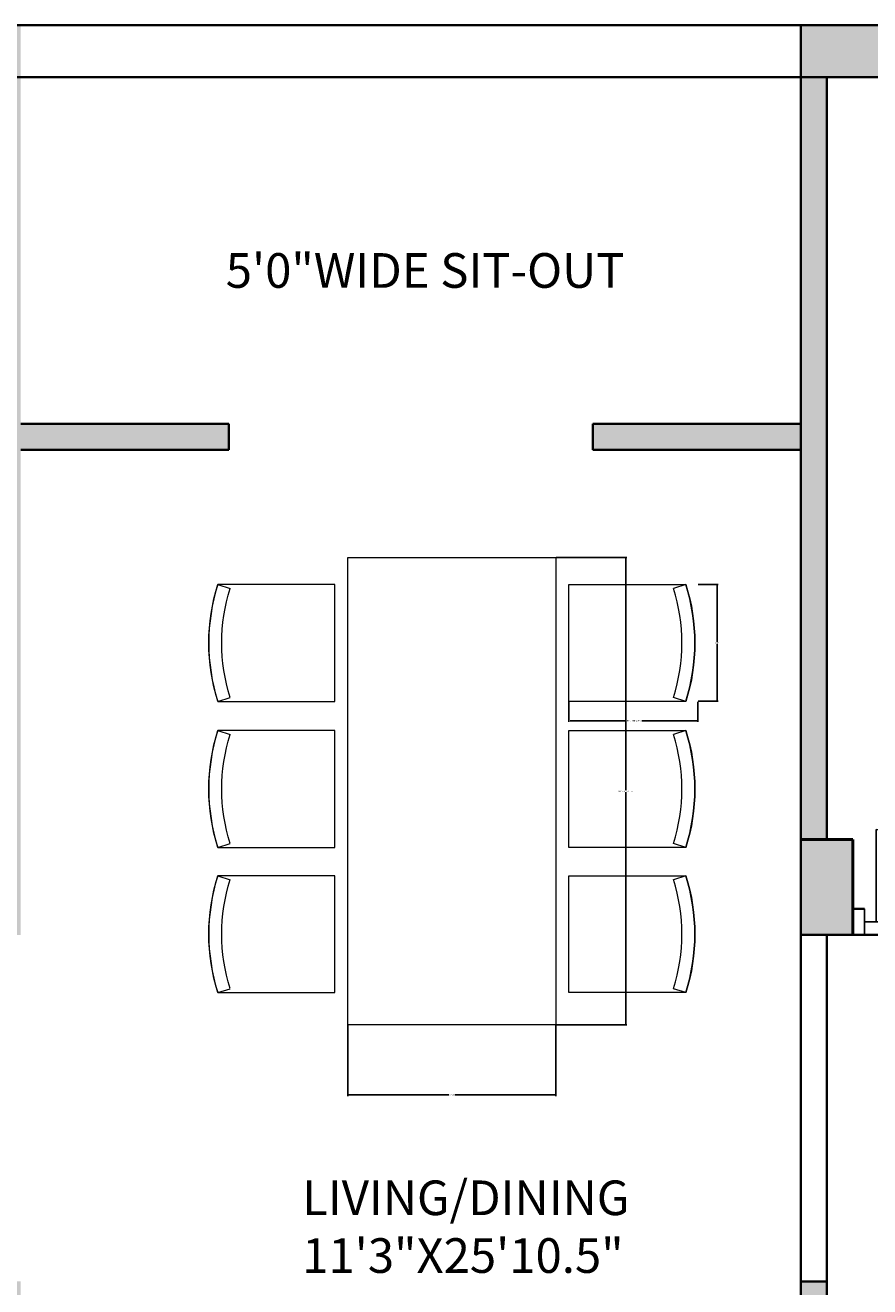
# Model space of a CAD drawing. Units: inches. Extents: x -28 to 485, y -861 to 54.
# Tile 12 of 14: x 162 to 308, y -208 to 10. Entities that reach past the tile are written whole.
import ezdxf

# ---------------------------------------------------------------- set-up
doc = ezdxf.new("R2010")
doc.units = ezdxf.units.IN
doc.header["$MEASUREMENT"] = 0
for name, color, linetype, lineweight in [('A-ANNO-DIMS', 2, 'Continuous', 18), ('A-AREA-IDEN', 7, 'Continuous', 18), ('A-COLS', 7, 'Continuous', 50), ('A-COLS-PATT', 8, 'Continuous', 13), ('A-DOOR', 3, 'Continuous', 25), ('A-FURN', 8, 'Continuous', 13), ('A-WALL', 7, 'Continuous', 35), ('A-WALL-PATT', 34, 'Continuous', 13)]:
    doc.layers.add(name, color=color, linetype=linetype, lineweight=lineweight)
doc.styles.get("Standard").update_dxf_attribs({"font": 'arial.ttf'})
doc.dimstyles.get("Standard").update_dxf_attribs({"dimtxt": 0.18, "dimasz": 0.18, "dimexe": 0.18, "dimexo": 0.0625, "dimgap": 0.09, "dimtad": 0, "dimtih": 1, "dimtoh": 1, "dimdec": 0, "dimzin": 0, "dimdsep": 46, "dimlunit": 3, "dimtxsty": 'Standard', "dimcen": 0.09, "dimadec": 0, "dimazin": 0, "dimtfac": 1, "dimtdec": 0, "dimtofl": 0, "dimtmove": 0, "dimatfit": 3, "dimfxl": 1, "dimtolj": 1, "dimtzin": 0, "dimarcsym": 0})

# ---------------------------------------------------------------- blocks, each defined once
blk = doc.blocks.new('CHAIR-DINING')
for p, q in [((20.22, 20.23), (18.08, 19.55)), ((20.22, 0), (18.08, 0.68))]:
    blk.add_line(p, q)
blk.add_lwpolyline([(20.23, 0), (0, 0), (0, 20.23), (20.23, 20.23, -0.153703), (20.23, 0)], format="xyb")
for radius in [33.37, 31.13]:
    blk.add_arc((-11.59, 10.12), radius, 342.3544, 17.6456)
blk = doc.blocks.new('TABLE-DINING-RECT')
blk.add_lwpolyline([(0, 80.93), (35.97, 80.93), (35.97, 0), (0, 0)], close=True)
blk = doc.blocks.new('DOOR-SWING-NARROW')
for p, q in [((17, 2.25), (17, 18.25)), ((18, 2.25), (18, 18.25)), ((0, 2.25), (0, 4.5)), ((20, 4.5), (20, 0)), ((0, 2.25), (0, 0)), ((0, 2.25), (2, 2.25)), ((17, 2.25), (18, 2.25)), ((20, 2.25), (18, 2.25))]:
    blk.add_line(p, q)
blk.add_arc((18, 2.25), 16, 90, 180)
blk = doc.blocks.new('*D18')
at = {"layer": 'A-ANNO-DIMS', "color": 0, "lineweight": -2, "transparency": 16777216}
for p, q in [((255.64, -107), (255.64, -110.46)), ((277.95, -107), (277.95, -110.46)), ((255.82, -110.28), (265.37, -110.28)), ((277.77, -110.28), (268.22, -110.28))]:
    blk.add_line(p, q, dxfattribs=at)
at = {"layer": 'A-ANNO-DIMS', "color": 0, "transparency": 16777216}
for points in [[(255.82, -110.25), (255.82, -110.31), (255.64, -110.28)], [(277.77, -110.25), (277.77, -110.31), (277.95, -110.28)]]:
    blk.add_solid(points, dxfattribs=at)
at = {"layer": 'Defpoints', "color": 0, "transparency": 16777216}
for p in [(255.64, -106.93), (277.95, -106.93), (277.95, -110.28)]:
    blk.add_point(p, dxfattribs=at)
at = {"layer": 'A-ANNO-DIMS', "color": 0, "transparency": 16777216, "insert": (266.8, -110.28), "char_height": 0.18, "attachment_point": 5}
blk.add_mtext('\\A1;DINING CHAIR 22 TYP.', dxfattribs=at)
blk = doc.blocks.new('*D19')
at = {"layer": 'A-ANNO-DIMS', "color": 0, "lineweight": -2, "transparency": 16777216}
for p, q in [((278.01, -86.7), (281.48, -86.7)), ((281.3, -86.88), (281.3, -96.63)), ((281.3, -106.75), (281.3, -97)), ((278.01, -106.93), (281.48, -106.93))]:
    blk.add_line(p, q, dxfattribs=at)
at = {"layer": 'A-ANNO-DIMS', "color": 0, "transparency": 16777216}
for points in [[(281.27, -86.88), (281.33, -86.88), (281.3, -86.7)], [(281.27, -106.75), (281.33, -106.75), (281.3, -106.93)]]:
    blk.add_solid(points, dxfattribs=at)
at = {"layer": 'Defpoints', "color": 0, "transparency": 16777216}
for p in [(277.95, -86.7), (281.3, -86.7), (277.95, -106.93)]:
    blk.add_point(p, dxfattribs=at)
at = {"layer": 'A-ANNO-DIMS', "color": 0, "transparency": 16777216, "insert": (281.3, -96.82), "char_height": 0.18, "attachment_point": 5}
blk.add_mtext('\\A1;20 TYP.', dxfattribs=at)
blk = doc.blocks.new('*D42')
at = {"layer": 'A-ANNO-DIMS', "color": 0, "lineweight": -2, "transparency": 16777216}
for p, q in [((253.42, -82.02), (265.67, -82.02)), ((265.49, -82.2), (265.49, -122.3)), ((265.49, -162.77), (265.49, -122.67)), ((253.42, -162.95), (265.67, -162.95))]:
    blk.add_line(p, q, dxfattribs=at)
at = {"layer": 'A-ANNO-DIMS', "color": 0, "transparency": 16777216}
for points in [[(265.46, -82.2), (265.52, -82.2), (265.49, -82.02)], [(265.46, -162.77), (265.52, -162.77), (265.49, -162.95)]]:
    blk.add_solid(points, dxfattribs=at)
at = {"layer": 'Defpoints', "color": 0, "transparency": 16777216}
for p in [(253.35, -82.02), (265.49, -82.02), (253.35, -162.95)]:
    blk.add_point(p, dxfattribs=at)
at = {"layer": 'A-ANNO-DIMS', "color": 0, "transparency": 16777216, "insert": (265.49, -122.48), "char_height": 0.18, "attachment_point": 5}
blk.add_mtext('\\A1;DINING TABLE 81 TYP.', dxfattribs=at)
blk = doc.blocks.new('*D43')
at = {"layer": 'A-ANNO-DIMS', "color": 0, "lineweight": -2, "transparency": 16777216}
for p, q in [((217.38, -163.01), (217.38, -175.27)), ((253.35, -163.01), (253.35, -175.27)), ((217.56, -175.09), (234.84, -175.09)), ((253.17, -175.09), (235.9, -175.09))]:
    blk.add_line(p, q, dxfattribs=at)
at = {"layer": 'A-ANNO-DIMS', "color": 0, "transparency": 16777216}
for points in [[(217.56, -175.06), (217.56, -175.12), (217.38, -175.09)], [(253.17, -175.06), (253.17, -175.12), (253.35, -175.09)]]:
    blk.add_solid(points, dxfattribs=at)
at = {"layer": 'Defpoints', "color": 0, "transparency": 16777216}
for p in [(217.38, -162.95), (253.35, -162.95), (253.35, -175.09)]:
    blk.add_point(p, dxfattribs=at)
at = {"layer": 'A-ANNO-DIMS', "color": 0, "transparency": 16777216, "insert": (235.37, -175.09), "char_height": 0.18, "attachment_point": 5}
blk.add_mtext('\\A1;36 TYP.', dxfattribs=at)

msp = doc.modelspace()

# ---------------------------------------------------------------- hatches: boundary and pattern name
at = {"layer": 'A-COLS-PATT'}
h = msp.add_hatch(color=256, dxfattribs=at)
h.dxf.hatch_style = 1
h.paths.add_polyline_path([(36.285, 10.133), (15.285, 10.133), (15.285, 1.133), (36.285, 1.133)])
h.paths.add_polyline_path([(160.785, 10.133), (139.785, 10.133), (139.785, 1.133), (160.785, 1.133)])
h.paths.add_polyline_path([(316.785, 10.133), (295.785, 10.133), (295.785, 1.133), (316.785, 1.133)])
h.paths.add_polyline_path([(441.285, 10.133), (420.285, 10.133), (420.285, 1.133), (441.285, 1.133)])
h.paths.add_polyline_path([(441.285, -138.367), (432.285, -138.367), (420.285, -138.367), (420.285, -147.367), (441.285, -147.367)])
h.paths.add_polyline_path([(304.785, -130.867), (295.785, -130.867), (295.785, -147.367), (304.785, -147.367), (304.785, -142.867)])
h.paths.add_polyline_path([(160.785, -130.867), (151.785, -130.867), (151.785, -142.867), (151.785, -147.367), (160.785, -147.367)])
h.paths.add_polyline_path([(36.285, -138.367), (24.285, -138.367), (15.285, -138.367), (15.285, -147.367), (36.285, -147.367)])
h.paths.add_polyline_path([(36.285, -355.867), (15.285, -355.867), (15.285, -364.867), (36.285, -364.867)])
h.paths.add_polyline_path([(160.785, -355.867), (139.785, -355.867), (139.785, -364.867), (160.785, -364.867)])
h.paths.add_polyline_path([(316.785, -355.867), (300.285, -355.867), (295.785, -355.867), (295.785, -364.867), (316.785, -364.867)])
at = {"layer": 'A-WALL-PATT'}
h = msp.add_hatch(color=256, dxfattribs=at)
h.dxf.hatch_style = 1
h.paths.add_polyline_path([(160.785, -808.867), (160.785, -817.867), (295.785, -817.867), (295.785, -808.867)])
h.paths.add_polyline_path([(316.785, -817.867), (323.776, -817.867), (323.776, -808.867), (316.785, -808.867)])
h.paths.add_polyline_path([(420.285, -817.867), (420.285, -808.867), (383.776, -808.867), (383.776, -817.867)])
h.paths.add_polyline_path([(432.285, -808.867), (441.285, -808.867), (441.285, -702.966), (432.285, -702.966), (432.285, -708.367), (397.785, -708.367), (397.785, -710.617), (397.785, -712.867), (432.285, -712.867)])
h.paths.add_polyline_path([(300.285, -712.867), (329.285, -712.867), (329.285, -710.617), (329.285, -708.367), (295.785, -708.367), (295.785, -808.867), (300.285, -808.867)])
h.paths.add_polyline_path([(160.785, -698.867), (158.535, -698.867), (156.285, -698.867), (156.285, -808.867), (160.785, -808.867)])
h.paths.add_polyline_path([(36.285, -808.867), (36.285, -817.867), (79.721, -817.867), (79.721, -808.867)])
h.paths.add_polyline_path([(15.285, -808.867), (24.285, -808.867), (24.285, -739.09), (15.285, -739.09)])
h.paths.add_polyline_path([(24.285, -640.781), (15.285, -640.781), (15.285, -679.09), (24.285, -679.09), (24.285, -664.867), (89.285, -664.867), (89.285, -662.617), (89.285, -660.367), (24.285, -660.367)])
h.paths.add_polyline_path([(15.285, -616.781), (24.285, -616.781), (24.285, -600.367), (15.285, -600.367)])
h.paths.add_polyline_path([(36.285, -595.867), (36.285, -600.367), (123.285, -600.367), (123.285, -660.367), (117.285, -660.367), (117.285, -664.867), (156.285, -664.867), (156.285, -670.867), (160.785, -670.867), (160.785, -660.367), (127.785, -660.367), (127.785, -600.367), (129.785, -600.367), (129.785, -598.117), (129.785, -595.867)])
h.paths.add_polyline_path([(367.785, -664.867), (363.285, -664.867), (363.285, -708.367), (357.285, -708.367), (357.285, -712.867), (369.785, -712.867), (369.785, -708.367), (367.785, -708.367)])
h.paths.add_polyline_path([(432.285, -664.867), (432.285, -666.966), (441.285, -666.966), (441.285, -642.367), (432.285, -642.367), (432.285, -660.367), (328.785, -660.367), (328.785, -664.867), (363.285, -664.867)])
h.paths.add_polyline_path([(333.285, -600.367), (420.285, -600.367), (420.285, -595.867), (326.785, -595.867), (326.785, -600.367), (328.785, -600.367), (328.785, -630.367), (331.035, -630.367), (333.285, -630.367)])
h.paths.add_polyline_path([(441.285, -600.367), (432.285, -600.367), (432.285, -618.367), (441.285, -618.367)])
h.paths.add_polyline_path([(432.285, -591.367), (441.285, -591.367), (441.285, -547.793), (432.285, -547.793)])
h.paths.add_polyline_path([(295.785, -588.367), (300.238, -588.367), (300.285, -583.867), (300.285, -451.867), (295.785, -451.867)])
h.paths.add_polyline_path([(420.285, -451.867), (420.285, -442.867), (316.785, -442.867), (316.785, -451.867)])
h.paths.add_polyline_path([(432.285, -487.793), (441.285, -487.793), (441.285, -451.867), (432.285, -451.867)])
h.paths.add_polyline_path([(432.285, -442.867), (441.285, -442.867), (441.285, -364.867), (432.285, -364.867)])
h.paths.add_polyline_path([(261.785, -451.867), (261.785, -447.367), (261.785, -444.758), (261.785, -442.867), (160.785, -442.867), (160.785, -451.867)])
h.paths.add_polyline_path([(139.785, -451.867), (139.785, -442.867), (36.285, -442.867), (36.285, -451.867)])
h.paths.add_polyline_path([(15.285, -491.617), (24.285, -491.617), (24.285, -451.867), (15.285, -451.867)])
h.paths.add_polyline_path([(24.285, -551.617), (15.285, -551.617), (15.285, -591.367), (24.285, -591.367)])
h.paths.add_polyline_path([(160.785, -451.867), (156.285, -451.867), (156.285, -588.367), (160.785, -588.367)])
h.paths.add_polyline_path([(139.785, -364.867), (139.785, -355.867), (36.285, -355.867), (36.285, -364.867)])
h.paths.add_polyline_path([(24.285, -364.867), (15.285, -364.867), (15.285, -373.867), (24.285, -373.867)])
h.paths.add_polyline_path([(15.285, -433.867), (15.285, -442.867), (24.285, -442.867), (24.285, -433.867)])
h.paths.add_polyline_path([(261.785, -364.867), (261.785, -360.367), (261.785, -355.867), (160.785, -355.867), (160.785, -364.867)])
h.paths.add_polyline_path([(295.785, -355.867), (289.785, -355.867), (289.785, -364.867), (295.785, -364.867)])
h.paths.add_polyline_path([(295.785, -355.867), (300.285, -355.867), (300.285, -259.867), (333.285, -259.867), (333.285, -257.617), (333.285, -255.367), (300.285, -255.367), (300.285, -207.367), (295.785, -207.367)])
h.paths.add_polyline_path([(420.285, -364.867), (420.285, -355.867), (316.785, -355.867), (316.785, -364.867)])
h.paths.add_polyline_path([(24.285, -311.192), (15.285, -311.192), (15.285, -355.867), (24.285, -355.867)])
h.paths.add_polyline_path([(24.285, -211.867), (54.144, -211.867), (54.144, -207.367), (24.285, -207.367), (24.285, -187.772), (15.285, -187.772), (15.285, -251.192), (24.285, -251.192)])
h.paths.add_polyline_path([(82.144, -207.367), (82.144, -209.617), (82.144, -211.867), (127.785, -211.867), (127.785, -147.367), (129.785, -147.367), (129.785, -145.117), (129.785, -142.867), (36.285, -142.867), (36.285, -147.367), (123.285, -147.367), (123.285, -207.367)])
h.paths.add_polyline_path([(160.785, -207.367), (156.285, -207.367), (156.285, -355.867), (160.785, -355.867)])
h.paths.add_polyline_path([(24.285, 1.133), (15.285, 1.133), (15.285, -54.408), (24.285, -54.408)])
h.paths.add_polyline_path([(36.285, 10.133), (36.285, 1.133), (70.235, 1.133), (70.235, 10.133)])
h.paths.add_polyline_path([(15.285, -138.367), (24.285, -138.367), (24.285, -114.408), (15.285, -114.408)])
h.paths.add_polyline_path([(24.285, -147.367), (15.285, -147.367), (15.285, -163.772), (24.285, -163.772)])
h.paths.add_polyline_path([(156.285, -130.867), (160.785, -130.867), (160.785, 1.133), (156.285, 1.133)])
h.paths.add_polyline_path([(130.235, 1.133), (139.785, 1.133), (139.785, 10.133), (130.235, 10.133)])
h.paths.add_polyline_path([(316.785, 10.133), (316.785, 1.133), (328.097, 1.133), (328.097, 10.133)])
h.paths.add_polyline_path([(300.285, 1.133), (295.785, 1.133), (295.785, -130.867), (300.285, -130.867)])
h.paths.add_polyline_path([(420.285, -147.367), (420.285, -142.867), (326.785, -142.867), (326.785, -145.117), (326.785, -147.367), (328.785, -147.367), (328.785, -177.367), (331.035, -177.367), (333.285, -177.367), (333.285, -147.367)])
h.paths.add_polyline_path([(333.285, -207.367), (333.285, -205.367), (328.785, -205.367), (328.785, -211.867), (363.285, -211.867), (363.285, -255.367), (361.285, -255.367), (361.285, -259.867), (369.785, -259.867), (369.785, -255.367), (367.785, -255.367), (367.785, -211.867), (432.285, -211.867), (432.285, -214.893), (441.285, -214.893), (441.285, -188.008), (432.285, -188.008), (432.285, -207.367)])
h.paths.add_polyline_path([(441.285, -250.893), (432.285, -250.893), (432.285, -255.367), (397.785, -255.367), (397.785, -257.617), (397.785, -259.867), (432.285, -259.867), (432.285, -355.867), (441.285, -355.867)])
h.paths.add_polyline_path([(432.285, -138.367), (441.285, -138.367), (441.285, -115.099), (432.285, -115.099)])
h.paths.add_polyline_path([(441.285, -147.367), (432.285, -147.367), (432.285, -164.008), (441.285, -164.008)])
h.paths.add_polyline_path([(420.285, 1.133), (420.285, 10.133), (388.097, 10.133), (388.097, 1.133)])
h.paths.add_polyline_path([(432.285, -55.099), (441.285, -55.099), (441.285, 1.133), (432.285, 1.133)])
h = msp.add_hatch(color=256, dxfattribs=at)
h.dxf.hatch_style = 1
h.paths.add_polyline_path([(196.785, -58.867), (160.785, -58.867), (160.785, -63.367), (196.785, -63.367)])
h.paths.add_polyline_path([(295.785, -58.867), (259.785, -58.867), (259.785, -63.367), (295.785, -63.367)])
h.paths.add_polyline_path([(196.785, -753.367), (160.785, -753.367), (160.785, -757.867), (196.785, -757.867)])
h.paths.add_polyline_path([(295.785, -753.367), (259.785, -753.367), (259.785, -757.867), (295.785, -757.867)])

# ---------------------------------------------------------------- linework, layer by layer
at = {"layer": 'A-COLS'}
for p, q in [((304.785, -130.867), (295.785, -130.867)), ((304.785, -142.867), (304.785, -130.867)), ((304.785, -147.367), (304.785, -142.867))]:
    msp.add_line(p, q, dxfattribs=at)
at = {"layer": 'A-WALL'}
for p, q in [((15.285, 10.133), (441.285, 10.133)), ((295.785, 10.133), (295.785, -364.867)), ((15.285, 1.133), (441.285, 1.133)), ((300.285, 1.133), (300.285, -130.867)), ((160.785, -58.867), (196.785, -58.867)), ((196.785, -58.867), (196.785, -63.367)), ((259.785, -58.867), (259.785, -63.367)), ((259.785, -58.867), (295.785, -58.867)), ((160.785, -63.367), (196.785, -63.367)), ((259.785, -63.367), (295.785, -63.367)), ((304.785, -142.867), (306.785, -142.867)), ((295.785, -147.367), (328.785, -147.367)), ((300.285, -147.367), (300.285, -255.367)), ((295.785, -207.367), (300.285, -207.367))]:
    msp.add_line(p, q, dxfattribs=at)

# ---------------------------------------------------------------- block references
at = {"layer": 'A-DOOR', "extrusion": (0, 0, -1), "zscale": -1}
msp.add_blockref('DOOR-SWING-NARROW', (-326.784, -147.367), dxfattribs=at)
at = {"layer": 'A-FURN'}
for name, p in [('TABLE-DINING-RECT', (217.384, -162.948)), ('CHAIR-DINING', (255.64, -106.933)), ('CHAIR-DINING', (255.64, -132.23)), ('CHAIR-DINING', (255.64, -157.362))]:
    msp.add_blockref(name, p, dxfattribs=at)
at = {"layer": 'A-FURN', "extrusion": (0, 0, -1), "zscale": -1}
for p in [(-215.097, -106.933), (-215.097, -132.23), (-215.097, -157.362)]:
    msp.add_blockref('CHAIR-DINING', p, dxfattribs=at)

# ---------------------------------------------------------------- texts
at = {"layer": 'A-AREA-IDEN', "char_height": 6, "attachment_point": 1}
for s, insert in [('5\'0"WIDE SIT-OUT', (196.25, -29.33)), ('LIVING/DINING\\P11\'3"X25\'10.5"', (209.474, -189.892))]:
    msp.add_mtext(s, dxfattribs=dict(at, insert=insert))

# ---------------------------------------------------------------- dimensions: what is measured, and where the dimension line sits
at = {"layer": 'A-ANNO-DIMS'}
for base, p1, p2, text, picture, middle in [((265.493, -82.016), (253.354, -162.948), (253.354, -82.016), 'DINING TABLE <> TYP.', '*D42', (265.493, -122.482)), ((281.298, -86.7), (277.951, -106.933), (277.951, -86.7), '<> TYP.', '*D19', (281.298, -96.816))]:
    dim = msp.add_linear_dim(base=base, p1=p1, p2=p2, angle=90, text=text, dimstyle='Standard', override={"dimdec": 0, "dimlfac": 1, "dimrnd": 0, "dimzin": 0, "dimdsep": 46, "dimlunit": 2}, dxfattribs=at)
    dim.commit()
    dim.dimension.update_dxf_attribs({"geometry": picture, "text_midpoint": middle})
for base, p1, p2, text, picture, middle in [((277.951, -110.28), (255.64, -106.933), (277.951, -106.933), 'DINING CHAIR <> TYP.', '*D18', (266.795, -110.28)), ((253.354, -175.088), (217.384, -162.948), (253.354, -162.948), '<> TYP.', '*D43', (235.369, -175.088))]:
    dim = msp.add_linear_dim(base=base, p1=p1, p2=p2, text=text, dimstyle='Standard', override={"dimdec": 0, "dimlfac": 1, "dimrnd": 0, "dimzin": 0, "dimdsep": 46, "dimlunit": 2}, dxfattribs=at)
    dim.commit()
    dim.dimension.update_dxf_attribs({"geometry": picture, "text_midpoint": middle})

doc.saveas('drawing.dxf')
